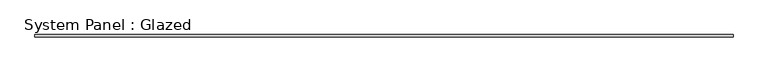
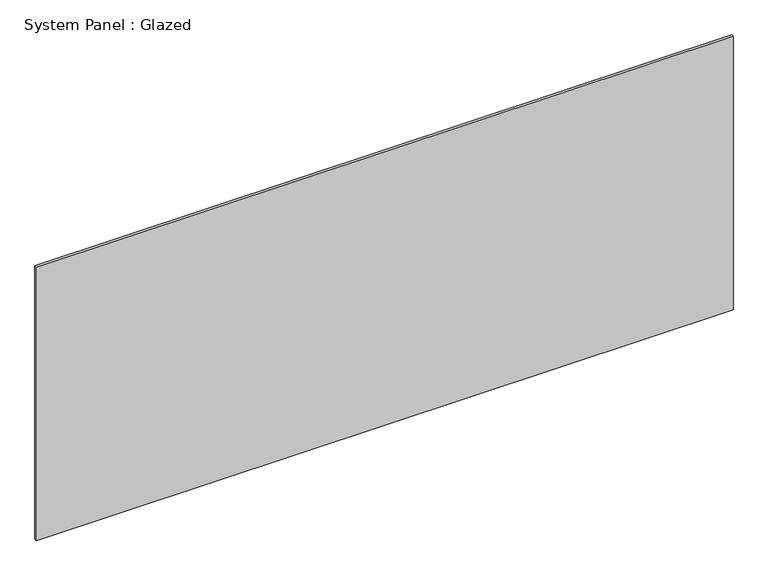
"""IFC4 building model written with IfcOpenShell, lengths in millimetres: plate geometry, System Panel : Glazed."""

from ifc_helpers import new_model, si_unit, origin, origin_with_axes, place, context, project, spatial, polyline, outline, extrude, source, transform, mapped, element, save


def system_panel_glazed_b550d99f(model_context):
    return source(origin(), model_context, "Body", "SweptSolid", [
        extrude(outline(polyline([(3670.3, 19.05), (-3670.3, 19.05), (-3670.3, 44.45), (3670.3, 44.45), (3670.3, 19.05)])), origin_with_axes(), (0.0, 0.0, 1.0), 3048.0),
    ])


if __name__ == "__main__":
    model = new_model("IFC4")
    model_context = context("Model", 3, world=origin())
    ifc_project = project(units=[si_unit("LENGTHUNIT", "METRE", prefix="MILLI")], contexts=[model_context])
    site = spatial("IfcSite", under=ifc_project)
    building = spatial("IfcBuilding", under=site)
    placement = place(None, origin())
    system_panel_glazed_shape = system_panel_glazed_b550d99f(model_context)
    element("IfcPlate", 1, ObjectType="System Panel : Glazed", at=placement, inside=building, context=model_context, shape_type="MappedRepresentation", body=[
        mapped(system_panel_glazed_shape, transform((0.0, 0.0, 0.0), x_axis=(1.0, 0.0, 0.0), y_axis=(0.0, 1.0, 0.0), z_axis=(0.0, 0.0, 1.0))),
    ])
    save(model, "model.ifc")

# Revit data of these elements
# Type "System Panel : Glazed"
#   Construction Type Id = "GSP4R"
#   Analytic Construction = "1/8 in Pilkington single glazing"
#   Visual Light Transmittance = 0.9
#   Solar Heat Gain Coefficient = 0.86
#   Heat Transfer Coefficient (U) = 1.18115 BTU/(h·ft²·°F)
# Element 1 (IfcPlate, "System Panel : Glazed")
#   Materials on its faces: "Glass"
# Materials
#   "Glass": class "Glass", colour RGB 0 128 192, transparency 0.75, Description = "Soda Lime Glass", Cost = 0
